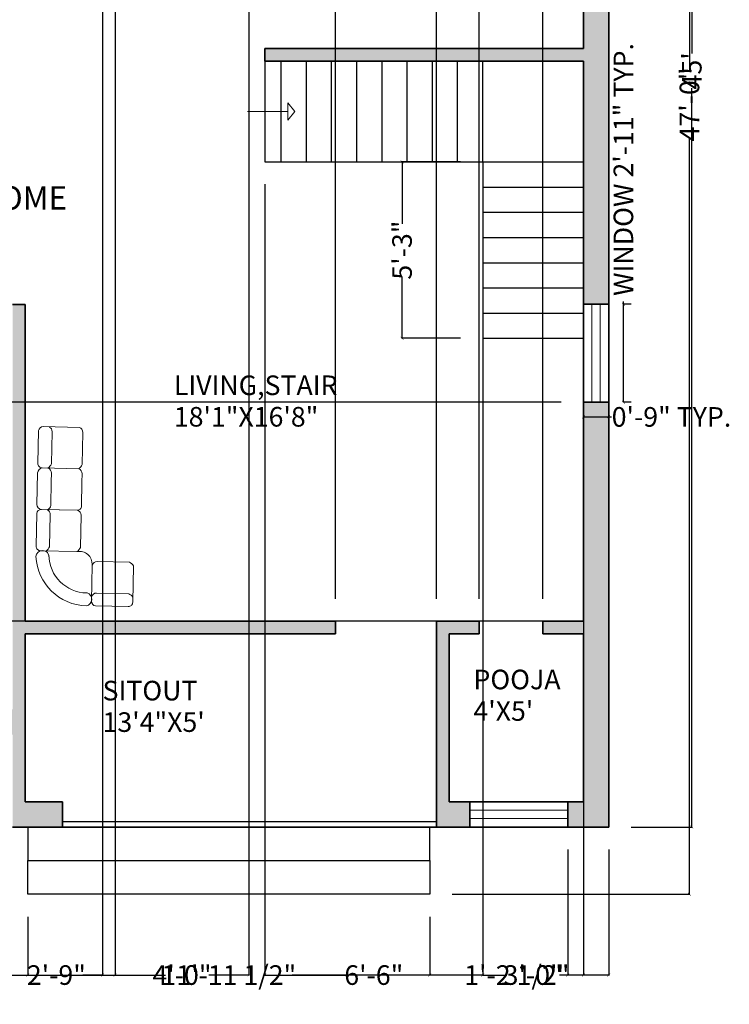
# Model space of a CAD drawing. Units: inches. Extents: x 98 to 545, y 56 to 703.
# Tile 2 of 4: x 292 to 545, y 56 to 408. Entities that reach past the tile are written whole.
import ezdxf

# ---------------------------------------------------------------- set-up
doc = ezdxf.new("R2010")
doc.units = ezdxf.units.IN
doc.header["$MEASUREMENT"] = 0
for name, color, linetype, lineweight in [('A-ANNO-DIMS', 2, 'Continuous', 18), ('A-ANNO-SYMB', 7, 'Continuous', 18), ('A-ANNO-TEXT', 7, 'Continuous', 25), ('A-AREA-IDEN', 7, 'Continuous', 25), ('A-FLOR-STRS', 7, 'Continuous', 25), ('A-GLAZ', 4, 'Continuous', 18), ('A-WALL', 7, 'Continuous', 35), ('Furniture', 7, 'Continuous', 15)]:
    doc.layers.add(name, color=color, linetype=linetype, lineweight=lineweight)
doc.layers.add('A-WALL-PATT', color=18, linetype='Continuous', lineweight=13, true_color=0x000000)
doc.styles.get("Standard").update_dxf_attribs({"font": 'arial.ttf'})
doc.dimstyles.get("Standard").update_dxf_attribs({"dimtxt": 7, "dimasz": 1, "dimexe": 0.183, "dimexo": 8, "dimgap": 0.09, "dimtad": 0, "dimdec": 4, "dimzin": 0, "dimdsep": 46, "dimlunit": 3, "dimtxsty": 'Standard', "dimblk": 'ARCHTICK', "dimcen": 0, "dimclrd": 253, "dimclre": 251, "dimadec": 0, "dimazin": 0, "dimtfac": 1, "dimtdec": 4, "dimtofl": 0, "dimtmove": 0, "dimatfit": 3, "dimfxl": 1, "dimtolj": 1, "dimtzin": 0, "dimarcsym": 0})

# ---------------------------------------------------------------- blocks, each defined once
blk = doc.blocks.new('_ArchTick')
at = {"color": 0, "linetype": 'ByBlock', "const_width": 0.15}
blk.add_lwpolyline([(-0.5, -0.5), (0.5, 0.5)], dxfattribs=at)
blk = doc.blocks.new('*D2')
at = {"layer": 'A-ANNO-DIMS', "color": 0, "lineweight": -2, "transparency": 16777216}
for p, q in [((510.36, 659.7), (532.23, 659.7)), ((532.04, 659.7), (532.04, 395.87)), ((532.04, 119.7), (532.04, 383.53)), ((510.36, 119.7), (532.23, 119.7))]:
    blk.add_line(p, q, dxfattribs=at)
at = {"layer": 'Defpoints', "color": 0, "transparency": 16777216}
for p in [(502.36, 659.7), (502.36, 119.7), (532.04, 119.7)]:
    blk.add_point(p, dxfattribs=at)
at = {"layer": 'A-ANNO-DIMS', "color": 0, "lineweight": -2, "transparency": 16777216}
for p, rotation in [((532.04, 659.7), 90), ((532.04, 119.7), 270)]:
    blk.add_blockref('_ArchTick', p, dxfattribs=dict(at, rotation=rotation))
at = {"layer": 'A-ANNO-DIMS', "color": 0, "transparency": 16777216, "insert": (532.04, 389.7), "char_height": 7, "attachment_point": 5, "rotation": 90}
blk.add_mtext("\\A1;45'", dxfattribs=at)
blk = doc.blocks.new('WIN-SASH-35IN')
for p, q in [((0, 35), (0, 0)), ((3, 35), (3, 0)), ((6, 35), (6, 0)), ((9, 0), (9, 35))]:
    blk.add_line(p, q)
blk = doc.blocks.new('*D11')
at = {"layer": 'A-ANNO-DIMS', "color": 253, "lineweight": -2, "transparency": 16777216}
for p, q in [((507.61, 306.39), (507.61, 307.39)), ((507.61, 271.39), (507.61, 306.39))]:
    blk.add_line(p, q, dxfattribs=at)
at = {"layer": 'A-ANNO-DIMS', "color": 251, "lineweight": -2, "transparency": 16777216}
for p, q in [((510.36, 306.39), (507.8, 306.39)), ((510.36, 271.39), (507.8, 271.39))]:
    blk.add_line(p, q, dxfattribs=at)
at = {"layer": 'Defpoints', "color": 0, "transparency": 16777216}
for p in [(502.36, 306.39), (507.61, 306.39), (502.36, 271.39)]:
    blk.add_point(p, dxfattribs=at)
at = {"layer": 'A-ANNO-DIMS', "color": 253, "lineweight": -2, "transparency": 16777216}
for p, rotation in [((507.61, 306.39), 90), ((507.61, 271.39), 270)]:
    blk.add_blockref('_ArchTick', p, dxfattribs=dict(at, rotation=rotation))
at = {"layer": 'A-ANNO-DIMS', "color": 0, "transparency": 16777216, "insert": (507.61, 354.48), "char_height": 7, "attachment_point": 5, "rotation": 90}
blk.add_mtext('\\A1;WINDOW 2\'-11" TYP.', dxfattribs=at)
blk = doc.blocks.new('*D12')
at = {"layer": 'A-ANNO-DIMS', "color": 253, "lineweight": -2, "transparency": 16777216}
for p, q in [((493.36, 266.14), (502.36, 266.14)), ((502.36, 266.14), (503.36, 266.14))]:
    blk.add_line(p, q, dxfattribs=at)
at = {"layer": 'A-ANNO-DIMS', "color": 251, "lineweight": -2, "transparency": 16777216}
for p, q in [((493.36, 263.39), (493.36, 265.95)), ((502.36, 263.39), (502.36, 265.95))]:
    blk.add_line(p, q, dxfattribs=at)
at = {"layer": 'Defpoints', "color": 0, "transparency": 16777216}
for p in [(493.36, 271.39), (502.36, 271.39), (502.36, 266.14)]:
    blk.add_point(p, dxfattribs=at)
at = {"layer": 'A-ANNO-DIMS', "color": 253, "lineweight": -2, "transparency": 16777216, "rotation": 180}
blk.add_blockref('_ArchTick', (493.36, 266.14), dxfattribs=at)
at = {"layer": 'A-ANNO-DIMS', "color": 253, "lineweight": -2, "transparency": 16777216}
blk.add_blockref('_ArchTick', (502.36, 266.14), dxfattribs=at)
at = {"layer": 'A-ANNO-DIMS', "color": 0, "transparency": 16777216, "insert": (524.79, 266.14), "char_height": 7, "attachment_point": 5}
blk.add_mtext('\\A1;0\'-9" TYP.', dxfattribs=at)
blk = doc.blocks.new('*D17')
at = {"layer": 'A-ANNO-DIMS', "color": 251, "lineweight": -2, "transparency": 16777216}
for p, q in [((510.36, 659.7), (531.4, 659.7)), ((446.43, 95.7), (531.4, 95.7))]:
    blk.add_line(p, q, dxfattribs=at)
at = {"layer": 'A-ANNO-DIMS', "color": 253, "lineweight": -2, "transparency": 16777216}
for p, q in [((531.21, 659.7), (531.21, 389.95)), ((531.21, 95.7), (531.21, 365.44))]:
    blk.add_line(p, q, dxfattribs=at)
at = {"layer": 'Defpoints', "color": 0, "transparency": 16777216}
for p in [(502.36, 659.7), (531.21, 659.7), (438.43, 95.7)]:
    blk.add_point(p, dxfattribs=at)
at = {"layer": 'A-ANNO-DIMS', "color": 253, "lineweight": -2, "transparency": 16777216}
for p, rotation in [((531.21, 659.7), 90), ((531.21, 95.7), 270)]:
    blk.add_blockref('_ArchTick', p, dxfattribs=dict(at, rotation=rotation))
at = {"layer": 'A-ANNO-DIMS', "color": 0, "transparency": 16777216, "insert": (531.21, 377.7), "char_height": 7, "attachment_point": 5, "rotation": 90}
blk.add_mtext('\\A1;47\'-0"', dxfattribs=at)
blk = doc.blocks.new('*D30')
at = {"layer": 'A-ANNO-DIMS', "color": 251, "lineweight": -2, "transparency": 16777216}
for p, q in [((487.75, 111.7), (487.75, 66.66)), ((502.36, 111.7), (502.36, 66.66))]:
    blk.add_line(p, q, dxfattribs=at)
at = {"layer": 'A-ANNO-DIMS', "color": 253, "lineweight": -2, "transparency": 16777216}
for p, q in [((487.75, 66.85), (486.75, 66.85)), ((502.36, 66.85), (487.75, 66.85))]:
    blk.add_line(p, q, dxfattribs=at)
at = {"layer": 'Defpoints', "color": 0, "transparency": 16777216}
for p in [(487.75, 119.7), (502.36, 119.7), (487.75, 66.85)]:
    blk.add_point(p, dxfattribs=at)
at = {"layer": 'A-ANNO-DIMS', "color": 253, "lineweight": -2, "transparency": 16777216, "rotation": 180}
blk.add_blockref('_ArchTick', (487.75, 66.85), dxfattribs=at)
at = {"layer": 'A-ANNO-DIMS', "color": 253, "lineweight": -2, "transparency": 16777216}
blk.add_blockref('_ArchTick', (502.36, 66.85), dxfattribs=at)
at = {"layer": 'A-ANNO-DIMS', "color": 0, "transparency": 16777216, "insert": (469.53, 66.85), "char_height": 7, "attachment_point": 5}
blk.add_mtext('\\A1;1\'-2 1/2"', dxfattribs=at)
blk = doc.blocks.new('*D33')
at = {"layer": 'A-ANNO-DIMS', "color": 251, "lineweight": -2, "transparency": 16777216}
for p, q in [((485.36, 271.39), (113.33, 271.39)), ((485.36, 193.2), (113.33, 193.2))]:
    blk.add_line(p, q, dxfattribs=at)
at = {"layer": 'A-ANNO-DIMS', "color": 253, "lineweight": -2, "transparency": 16777216}
for p, q in [((113.51, 271.39), (113.51, 241.7)), ((113.51, 193.2), (113.51, 222.88))]:
    blk.add_line(p, q, dxfattribs=at)
at = {"layer": 'Defpoints', "color": 0, "transparency": 16777216}
for p in [(493.36, 271.39), (113.51, 193.2), (493.36, 193.2)]:
    blk.add_point(p, dxfattribs=at)
at = {"layer": 'A-ANNO-DIMS', "color": 253, "lineweight": -2, "transparency": 16777216}
for p, rotation in [((113.51, 271.39), 90), ((113.51, 193.2), 270)]:
    blk.add_blockref('_ArchTick', p, dxfattribs=dict(at, rotation=rotation))
at = {"layer": 'A-ANNO-DIMS', "color": 0, "transparency": 16777216, "insert": (113.51, 232.29), "char_height": 7, "attachment_point": 5, "rotation": 90}
blk.add_mtext('\\A1;6\'-6"', dxfattribs=at)
blk = doc.blocks.new('*D34')
at = {"layer": 'A-ANNO-DIMS', "color": 251, "lineweight": -2, "transparency": 16777216}
for p, q in [((404.75, 201.2), (404.75, 688.73)), ((440.86, 201.2), (440.86, 688.73))]:
    blk.add_line(p, q, dxfattribs=at)
at = {"layer": 'A-ANNO-DIMS', "color": 253, "lineweight": -2, "transparency": 16777216}
for p, q in [((404.75, 688.55), (413.41, 688.55)), ((440.86, 688.55), (432.2, 688.55))]:
    blk.add_line(p, q, dxfattribs=at)
at = {"layer": 'Defpoints', "color": 0, "transparency": 16777216}
for p in [(440.86, 688.55), (404.75, 193.2), (440.86, 193.2)]:
    blk.add_point(p, dxfattribs=at)
at = {"layer": 'A-ANNO-DIMS', "color": 253, "lineweight": -2, "transparency": 16777216, "rotation": 180}
blk.add_blockref('_ArchTick', (404.75, 688.55), dxfattribs=at)
at = {"layer": 'A-ANNO-DIMS', "color": 253, "lineweight": -2, "transparency": 16777216}
blk.add_blockref('_ArchTick', (440.86, 688.55), dxfattribs=at)
at = {"layer": 'A-ANNO-DIMS', "color": 0, "transparency": 16777216, "insert": (422.81, 688.55), "char_height": 7, "attachment_point": 5}
blk.add_mtext('\\A1;3\'-0"', dxfattribs=at)
blk = doc.blocks.new('*D35')
at = {"layer": 'A-ANNO-DIMS', "color": 251, "lineweight": -2, "transparency": 16777216}
for p, q in [((456.13, 201.2), (456.13, 688.73)), ((478.77, 201.2), (478.77, 688.73))]:
    blk.add_line(p, q, dxfattribs=at)
at = {"layer": 'A-ANNO-DIMS', "color": 253, "lineweight": -2, "transparency": 16777216}
for p, q in [((456.13, 688.55), (478.77, 688.55)), ((478.77, 688.55), (479.77, 688.55))]:
    blk.add_line(p, q, dxfattribs=at)
at = {"layer": 'Defpoints', "color": 0, "transparency": 16777216}
for p in [(478.77, 688.55), (456.13, 193.2), (478.77, 193.2)]:
    blk.add_point(p, dxfattribs=at)
at = {"layer": 'A-ANNO-DIMS', "color": 253, "lineweight": -2, "transparency": 16777216, "rotation": 180}
blk.add_blockref('_ArchTick', (456.13, 688.55), dxfattribs=at)
at = {"layer": 'A-ANNO-DIMS', "color": 253, "lineweight": -2, "transparency": 16777216}
blk.add_blockref('_ArchTick', (478.77, 688.55), dxfattribs=at)
at = {"layer": 'A-ANNO-DIMS', "color": 0, "transparency": 16777216, "insert": (499.7, 688.55), "char_height": 7, "attachment_point": 5}
blk.add_mtext('\\A1;1\'-10 1/2"', dxfattribs=at)
blk = doc.blocks.new('*D36')
at = {"layer": 'A-ANNO-DIMS', "color": 251, "lineweight": -2, "transparency": 16777216}
for p, q in [((325.96, 518.2), (325.96, 66.66)), ((373.81, 518.2), (373.81, 66.66))]:
    blk.add_line(p, q, dxfattribs=at)
at = {"layer": 'A-ANNO-DIMS', "color": 253, "lineweight": -2, "transparency": 16777216}
for p, q in [((325.96, 66.85), (340.35, 66.85)), ((373.81, 66.85), (359.42, 66.85))]:
    blk.add_line(p, q, dxfattribs=at)
at = {"layer": 'Defpoints', "color": 0, "transparency": 16777216}
for p in [(325.96, 526.2), (373.81, 526.2), (373.81, 66.85)]:
    blk.add_point(p, dxfattribs=at)
at = {"layer": 'A-ANNO-DIMS', "color": 253, "lineweight": -2, "transparency": 16777216, "rotation": 180}
blk.add_blockref('_ArchTick', (325.96, 66.85), dxfattribs=at)
at = {"layer": 'A-ANNO-DIMS', "color": 253, "lineweight": -2, "transparency": 16777216}
blk.add_blockref('_ArchTick', (373.81, 66.85), dxfattribs=at)
at = {"layer": 'A-ANNO-DIMS', "color": 0, "transparency": 16777216, "insert": (349.89, 66.85), "char_height": 7, "attachment_point": 5}
blk.add_mtext('\\A1;4\'-0"', dxfattribs=at)
blk = doc.blocks.new('*D37')
at = {"layer": 'A-ANNO-DIMS', "color": 251, "lineweight": -2, "transparency": 16777216}
for p, q in [((457.36, 286.2), (457.36, 66.66)), ((493.36, 286.2), (493.36, 66.66))]:
    blk.add_line(p, q, dxfattribs=at)
at = {"layer": 'A-ANNO-DIMS', "color": 253, "lineweight": -2, "transparency": 16777216}
for p, q in [((457.36, 66.85), (465.97, 66.85)), ((493.36, 66.85), (484.76, 66.85))]:
    blk.add_line(p, q, dxfattribs=at)
at = {"layer": 'Defpoints', "color": 0, "transparency": 16777216}
for p in [(457.36, 294.2), (493.36, 294.2), (493.36, 66.85)]:
    blk.add_point(p, dxfattribs=at)
at = {"layer": 'A-ANNO-DIMS', "color": 253, "lineweight": -2, "transparency": 16777216, "rotation": 180}
blk.add_blockref('_ArchTick', (457.36, 66.85), dxfattribs=at)
at = {"layer": 'A-ANNO-DIMS', "color": 253, "lineweight": -2, "transparency": 16777216}
blk.add_blockref('_ArchTick', (493.36, 66.85), dxfattribs=at)
at = {"layer": 'A-ANNO-DIMS', "color": 0, "transparency": 16777216, "insert": (475.36, 66.85), "char_height": 7, "attachment_point": 5}
blk.add_mtext('\\A1;3\'-0"', dxfattribs=at)
blk = doc.blocks.new('*D38')
at = {"layer": 'A-ANNO-DIMS', "color": 251, "lineweight": -2, "transparency": 16777216}
for p, q in [((379.48, 349.2), (379.48, 66.66)), ((457.36, 349.2), (457.36, 66.66))]:
    blk.add_line(p, q, dxfattribs=at)
at = {"layer": 'A-ANNO-DIMS', "color": 253, "lineweight": -2, "transparency": 16777216}
for p, q in [((379.48, 66.85), (409.01, 66.85)), ((457.36, 66.85), (427.83, 66.85))]:
    blk.add_line(p, q, dxfattribs=at)
at = {"layer": 'Defpoints', "color": 0, "transparency": 16777216}
for p in [(379.48, 357.2), (457.36, 357.2), (457.36, 66.85)]:
    blk.add_point(p, dxfattribs=at)
at = {"layer": 'A-ANNO-DIMS', "color": 253, "lineweight": -2, "transparency": 16777216, "rotation": 180}
blk.add_blockref('_ArchTick', (379.48, 66.85), dxfattribs=at)
at = {"layer": 'A-ANNO-DIMS', "color": 253, "lineweight": -2, "transparency": 16777216}
blk.add_blockref('_ArchTick', (457.36, 66.85), dxfattribs=at)
at = {"layer": 'A-ANNO-DIMS', "color": 0, "transparency": 16777216, "insert": (418.42, 66.85), "char_height": 7, "attachment_point": 5}
blk.add_mtext('\\A1;6\'-6"', dxfattribs=at)
blk = doc.blocks.new('*D39')
at = {"layer": 'A-ANNO-DIMS', "color": 251, "lineweight": -2, "transparency": 16777216}
for p, q in [((449.36, 357.2), (428.33, 357.2)), ((449.36, 294.2), (428.33, 294.2))]:
    blk.add_line(p, q, dxfattribs=at)
at = {"layer": 'A-ANNO-DIMS', "color": 253, "lineweight": -2, "transparency": 16777216}
for p, q in [((428.51, 357.2), (428.51, 335.09)), ((428.51, 294.2), (428.51, 316.3))]:
    blk.add_line(p, q, dxfattribs=at)
at = {"layer": 'Defpoints', "color": 0, "transparency": 16777216}
for p in [(428.51, 357.2), (457.36, 357.2), (457.36, 294.2)]:
    blk.add_point(p, dxfattribs=at)
at = {"layer": 'A-ANNO-DIMS', "color": 253, "lineweight": -2, "transparency": 16777216}
for p, rotation in [((428.51, 357.2), 90), ((428.51, 294.2), 270)]:
    blk.add_blockref('_ArchTick', p, dxfattribs=dict(at, rotation=rotation))
at = {"layer": 'A-ANNO-DIMS', "color": 0, "transparency": 16777216, "insert": (428.51, 325.7), "char_height": 7, "attachment_point": 5, "rotation": 90}
blk.add_mtext('\\A1;5\'-3"', dxfattribs=at)
blk = doc.blocks.new('*D42')
at = {"layer": 'A-ANNO-DIMS', "color": 251, "lineweight": -2, "transparency": 16777216}
for p, q in [((288.56, 558.2), (288.56, 66.66)), ((321.46, 558.2), (321.46, 66.66))]:
    blk.add_line(p, q, dxfattribs=at)
at = {"layer": 'A-ANNO-DIMS', "color": 253, "lineweight": -2, "transparency": 16777216}
for p, q in [((288.56, 66.85), (295.56, 66.85)), ((321.46, 66.85), (314.46, 66.85))]:
    blk.add_line(p, q, dxfattribs=at)
at = {"layer": 'Defpoints', "color": 0, "transparency": 16777216}
for p in [(288.56, 566.2), (321.46, 566.2), (321.46, 66.85)]:
    blk.add_point(p, dxfattribs=at)
at = {"layer": 'A-ANNO-DIMS', "color": 253, "lineweight": -2, "transparency": 16777216, "rotation": 180}
blk.add_blockref('_ArchTick', (288.56, 66.85), dxfattribs=at)
at = {"layer": 'A-ANNO-DIMS', "color": 253, "lineweight": -2, "transparency": 16777216}
blk.add_blockref('_ArchTick', (321.46, 66.85), dxfattribs=at)
at = {"layer": 'A-ANNO-DIMS', "color": 0, "transparency": 16777216, "insert": (305.01, 66.85), "char_height": 7, "attachment_point": 5}
blk.add_mtext('\\A1;2\'-9"', dxfattribs=at)
blk = doc.blocks.new('*D43')
at = {"layer": 'A-ANNO-DIMS', "color": 251, "lineweight": -2, "transparency": 16777216}
for p, q in [((294.81, 87.7), (294.81, 66.66)), ((438.43, 87.7), (438.43, 66.66))]:
    blk.add_line(p, q, dxfattribs=at)
at = {"layer": 'A-ANNO-DIMS', "color": 253, "lineweight": -2, "transparency": 16777216}
for p, q in [((294.81, 66.85), (343.96, 66.85)), ((438.43, 66.85), (389.28, 66.85))]:
    blk.add_line(p, q, dxfattribs=at)
at = {"layer": 'Defpoints', "color": 0, "transparency": 16777216}
for p in [(294.81, 95.7), (438.43, 95.7), (438.43, 66.85)]:
    blk.add_point(p, dxfattribs=at)
at = {"layer": 'A-ANNO-DIMS', "color": 253, "lineweight": -2, "transparency": 16777216, "rotation": 180}
blk.add_blockref('_ArchTick', (294.81, 66.85), dxfattribs=at)
at = {"layer": 'A-ANNO-DIMS', "color": 253, "lineweight": -2, "transparency": 16777216}
blk.add_blockref('_ArchTick', (438.43, 66.85), dxfattribs=at)
at = {"layer": 'A-ANNO-DIMS', "color": 0, "transparency": 16777216, "insert": (366.62, 66.85), "char_height": 7, "attachment_point": 5}
blk.add_mtext('\\A1;11\'-11 1/2"', dxfattribs=at)
blk = doc.blocks.new('*D47')
at = {"layer": 'A-ANNO-DIMS', "color": 251, "lineweight": -2, "transparency": 16777216}
for p, q in [((271.36, 409.7), (271.36, 688.73)), ((275.86, 409.7), (275.86, 688.73))]:
    blk.add_line(p, q, dxfattribs=at)
at = {"layer": 'A-ANNO-DIMS', "color": 253, "lineweight": -2, "transparency": 16777216}
for p, q in [((271.36, 688.55), (275.86, 688.55)), ((275.86, 688.55), (276.86, 688.55))]:
    blk.add_line(p, q, dxfattribs=at)
at = {"layer": 'Defpoints', "color": 0, "transparency": 16777216}
for p in [(275.86, 688.55), (271.36, 401.7), (275.86, 401.7)]:
    blk.add_point(p, dxfattribs=at)
at = {"layer": 'A-ANNO-DIMS', "color": 253, "lineweight": -2, "transparency": 16777216, "rotation": 180}
blk.add_blockref('_ArchTick', (271.36, 688.55), dxfattribs=at)
at = {"layer": 'A-ANNO-DIMS', "color": 253, "lineweight": -2, "transparency": 16777216}
blk.add_blockref('_ArchTick', (275.86, 688.55), dxfattribs=at)
at = {"layer": 'A-ANNO-DIMS', "color": 0, "transparency": 16777216, "insert": (294.41, 688.55), "char_height": 7, "attachment_point": 5}
blk.add_mtext('\\A1;0\'-4 1/2"', dxfattribs=at)

msp = doc.modelspace()

# ---------------------------------------------------------------- hatches: boundary and pattern name
at = {"layer": 'A-WALL-PATT'}
h = msp.add_hatch(color=256, dxfattribs=at)
h.dxf.hatch_style = 1
h.paths.add_polyline_path([(173.39577, 659.69681), (142.36469, 659.69681), (142.36469, 612.44216), (151.36469, 612.44216), (151.36469, 650.69681), (173.39577, 650.69681)])
h.paths.add_polyline_path([(282.86266, 659.69681), (220.39577, 659.69681), (220.39577, 650.69681), (271.36469, 650.69681), (271.36469, 566.19681), (275.86469, 566.19681), (288.55623, 566.19681), (288.55623, 570.69681), (275.86469, 570.69681), (275.86469, 650.69681), (282.86266, 650.69681)])
h.paths.add_polyline_path([(358.82163, 659.69681), (312.86266, 659.69681), (312.86266, 650.69681), (321.46469, 650.69681), (321.46469, 570.69681), (321.46469, 566.19681), (321.46469, 530.69681), (321.46469, 526.19681), (325.96469, 526.19681), (325.96469, 530.69681), (325.96469, 650.69681), (358.82163, 650.69681)])
h.paths.add_polyline_path([(451.98971, 659.69681), (405.82163, 659.69681), (405.82163, 650.69681), (435.16469, 650.69681), (435.16469, 570.08746), (439.66469, 570.08746), (439.66469, 650.69681), (451.98971, 650.69681)])
h.paths.add_polyline_path([(502.36469, 659.69681), (481.98971, 659.69681), (481.98971, 650.69681), (493.36469, 650.69681), (493.36469, 614.57752), (502.36469, 614.57752)])
h.paths.add_polyline_path([(502.36469, 579.57752), (493.36469, 579.57752), (493.36469, 530.69681), (439.66469, 530.69681), (435.16469, 530.69681), (373.81242, 530.69681), (373.81242, 526.19681), (493.36469, 526.19681), (493.36469, 480.62471), (502.36469, 480.62471)])
h.paths.add_polyline_path([(502.36469, 445.62471), (493.36469, 445.62471), (493.36469, 406.19681), (493.36469, 401.69681), (493.36469, 397.69681), (379.47742, 397.69681), (379.47742, 393.19681), (493.36469, 393.19681), (493.36469, 306.38501), (502.36469, 306.38501)])
h.paths.add_polyline_path([(502.36469, 271.385), (493.36469, 271.385), (493.36469, 193.19681), (478.76571, 193.19681), (478.76571, 188.69681), (493.36469, 188.69681), (493.36469, 128.69681), (487.75103, 128.69681), (487.75103, 119.69681), (502.36469, 119.69681)])
h.paths.add_polyline_path([(452.75103, 128.69681), (445.36469, 128.69681), (445.36469, 188.69681), (456.12508, 188.69681), (456.12508, 193.19681), (440.86469, 193.19681), (440.86469, 119.69681), (452.75103, 119.69681)])
h.paths.add_polyline_path([(307.21941, 128.69681), (293.86469, 128.69681), (293.86469, 188.69681), (404.74827, 188.69681), (404.74827, 193.19681), (293.86469, 193.19681), (293.86469, 306.29681), (289.36469, 306.29681), (289.36469, 119.69681), (307.21941, 119.69681)])
h.paths.add_polyline_path([(289.36469, 161.69681), (238.02122, 161.69681), (238.02122, 152.69681), (289.36469, 152.69681)])
h.paths.add_polyline_path([(191.02122, 161.69681), (151.36469, 161.69681), (151.36469, 191.65928), (142.36469, 191.65928), (142.36469, 152.69681), (151.36469, 152.69681), (191.02122, 152.69681)])
h.paths.add_polyline_path([(151.36469, 306.29681), (151.36469, 308.54862), (142.36469, 308.54862), (142.36469, 238.65928), (151.36469, 238.65928)])
h.paths.add_polyline_path([(230.26469, 401.69681), (230.26469, 406.19681), (182.81458, 406.19681), (182.81458, 401.69681), (225.76469, 401.69681), (225.76469, 358.49681), (151.36469, 358.49681), (151.36469, 368.55378), (142.36469, 368.55378), (142.36469, 338.54862), (151.36469, 338.54862), (151.36469, 353.99681), (225.76469, 353.99681), (225.76469, 310.79681), (180.84919, 310.79681), (180.84919, 306.29681), (230.26469, 306.29681)])
h.paths.add_polyline_path([(151.36469, 442.07867), (142.36469, 442.07867), (142.36469, 398.55378), (151.36469, 398.55378), (151.36469, 401.69681)])
h.paths.add_polyline_path([(151.36469, 526.19681), (271.36469, 526.19681), (271.36469, 406.19681), (271.36469, 401.69681), (275.86469, 401.69681), (275.86469, 406.19681), (275.86469, 526.19681), (275.86469, 530.69681), (271.36469, 530.69681), (151.36469, 530.69681), (151.36469, 565.44216), (142.36469, 565.44216), (142.36469, 489.07867), (151.36469, 489.07867)])

# ---------------------------------------------------------------- linework, layer by layer
at = {"layer": 'A-ANNO-SYMB'}
for p, q in [((390.21777, 375.19681), (387.6515, 378.31614)), ((387.6515, 378.31614), (387.6515, 375.19681)), ((373.3537, 375.19681), (387.6515, 375.19681)), ((390.21777, 375.19681), (387.6515, 372.07747)), ((387.6515, 372.07747), (387.6515, 375.19681))]:
    msp.add_line(p, q, dxfattribs=at)
at = {"layer": 'A-FLOR-STRS'}
for p, q in [((379.47742, 393.19681), (379.47742, 357.19681)), ((385.36469, 357.19681), (385.36469, 393.19681)), ((394.36469, 357.19681), (394.36469, 393.19681)), ((403.36469, 357.19681), (403.36469, 393.19681)), ((412.36469, 357.19681), (412.36469, 393.19681)), ((421.36469, 357.19681), (421.36469, 393.19681)), ((430.36469, 357.19681), (430.36469, 393.19681)), ((439.36469, 357.19681), (439.36469, 393.19681)), ((448.36469, 357.19681), (448.36469, 393.19681)), ((457.36469, 357.19681), (457.36469, 393.19681)), ((379.47742, 357.19681), (493.36469, 357.19681)), ((457.36469, 357.19681), (457.36469, 294.19681)), ((457.36469, 348.19681), (493.36469, 348.19681)), ((457.36469, 339.19681), (493.36469, 339.19681)), ((457.36469, 330.19681), (493.36469, 330.19681)), ((457.36469, 321.19681), (493.36469, 321.19681)), ((457.36469, 312.19681), (493.36469, 312.19681)), ((457.36469, 303.19681), (493.36469, 303.19681)), ((457.36469, 294.19681), (493.36469, 294.19681)), ((294.80527, 119.69681), (294.80527, 107.69681)), ((307.21941, 121.69681), (440.86469, 121.69681)), ((438.43213, 107.69681), (438.43213, 119.69681)), ((294.80527, 107.69681), (438.43213, 107.69681)), ((294.80527, 95.69681), (294.80527, 107.69681)), ((438.43213, 107.69681), (438.43213, 95.69681)), ((438.43213, 95.69681), (294.80527, 95.69681))]:
    msp.add_line(p, q, dxfattribs=at)
at = {"layer": 'A-WALL'}
for p, q in [((502.36469, 119.69681), (502.36469, 659.69681)), ((493.36469, 406.19681), (493.36469, 526.19681)), ((493.36469, 401.69681), (493.36469, 406.19681)), ((493.36469, 397.69681), (493.36469, 401.69681)), ((379.47742, 397.69681), (493.36469, 397.69681)), ((379.47742, 397.69681), (379.47742, 393.19681)), ((379.47742, 393.19681), (493.36469, 393.19681)), ((493.36469, 193.19681), (493.36469, 393.19681)), ((293.86469, 306.29681), (289.36469, 306.29681)), ((293.86469, 306.29681), (293.86469, 193.19681)), ((502.36469, 306.38501), (493.36469, 306.38501)), ((493.36469, 271.385), (502.36469, 271.385)), ((293.86469, 193.19681), (404.74827, 193.19681)), ((404.74827, 193.19681), (404.74827, 188.69681)), ((440.86469, 119.69681), (440.86469, 193.19681)), ((440.86469, 193.19681), (456.12508, 193.19681)), ((456.12508, 188.69681), (456.12508, 193.19681)), ((478.76571, 188.69681), (478.76571, 193.19681)), ((478.76571, 193.19681), (493.36469, 193.19681)), ((293.86469, 188.69681), (404.74827, 188.69681)), ((293.86469, 188.69681), (293.86469, 128.69681)), ((445.36469, 128.69681), (445.36469, 188.69681)), ((445.36469, 188.69681), (456.12508, 188.69681)), ((478.76571, 188.69681), (493.36469, 188.69681)), ((493.36469, 128.69681), (493.36469, 188.69681)), ((293.86469, 128.69681), (307.21941, 128.69681)), ((307.21941, 128.69681), (307.21941, 119.69681)), ((445.36469, 128.69681), (493.36469, 128.69681)), ((452.75103, 128.69681), (452.75103, 119.69681)), ((487.75103, 119.69681), (487.75103, 128.69681)), ((289.36469, 119.69681), (502.36469, 119.69681))]:
    msp.add_line(p, q, dxfattribs=at)
at = {"layer": 'Furniture'}
for p, q in [((298.63616, 261.22932), (298.38808, 249.54981)), ((313.226, 262.3968), (300.27769, 262.67184)), ((303.22838, 249.37984), (303.4722, 260.85798)), ((314.21982, 249.14637), (314.46363, 260.62451)), ((298.31678, 246.19363), (298.07582, 234.84973)), ((299.96543, 247.97176), (312.97941, 247.62817)), ((302.98037, 234.54409), (303.16287, 243.13592)), ((303.16287, 243.13592), (303.22418, 246.02223)), ((313.97181, 234.31062), (314.15431, 242.90244)), ((314.15431, 242.90244), (314.21562, 245.78876)), ((299.51473, 233.07317), (312.39595, 232.79955)), ((312.59728, 232.79808), (299.64897, 233.07312)), ((298.00745, 231.63061), (297.75936, 219.95109)), ((302.59967, 219.78113), (302.84348, 231.25927)), ((313.5911, 219.54765), (313.83491, 231.02579)), ((299.33671, 218.37305), (312.35069, 218.02946)), ((331.09751, 214.23754), (319.61936, 214.48135)), ((317.84707, 213.24372), (317.57203, 200.29541)), ((332.6157, 212.99713), (332.27211, 199.98316)), ((316.02137, 203.27911), (315.86446, 203.28245)), ((317.60809, 201.99312), (317.60711, 201.94682)), ((330.85853, 202.98694), (319.38039, 203.23075)), ((319.01455, 198.65389), (330.69406, 198.4058))]:
    msp.add_line(p, q, dxfattribs=at)
for centre, radius, start, end in [((300.24336, 261.05566), 1.61655, 88.783137, 173.8328903), ((301.64015, 260.8969), 1.83246, 358.783137, 62.8574556), ((312.63158, 260.66342), 1.83246, 358.783137, 71.0719068), ((300.5577, 245.76926), 2.28074, 105.0511292, 169.276828), ((299.93328, 249.51699), 1.54556, 178.783137, 271.1919529), ((299.79157, 250.922), 3.76696, 305.666939, 335.8333646), ((301.29847, 246.06314), 1.92615, 358.783137, 69.0242602), ((310.783, 250.68853), 3.76696, 305.666939, 335.8333646), ((312.2899, 245.82966), 1.92615, 358.783137, 69.0242602), ((299.61464, 231.45694), 1.61655, 88.783137, 173.8328903), ((299.8456, 234.81214), 1.77017, 178.783137, 259.2272933), ((301.01143, 231.29818), 1.83246, 358.783137, 62.8574556), ((301.43729, 234.57609), 1.54341, 285.5408754, 358.8120982), ((312.42873, 234.34262), 1.54341, 268.783137, 358.8120982), ((312.00286, 231.06471), 1.83246, 358.783137, 71.0719068), ((300.03988, 216.14235), 2.34094, 356.795265, 176.795265), ((299.30456, 219.91827), 1.54556, 178.783137, 271.1919529), ((299.16285, 221.32329), 3.76696, 305.666939, 335.8333646), ((310.15428, 221.08981), 3.76696, 305.666939, 335.8333646), ((313.18783, 213.51232), 4.63077, 358.783137, 99.3837611), ((316.15958, 217.17584), 18.47811, 182.7701723, 268.7314166), ((316.15958, 217.17584), 13.89653, 181.6990742, 268.783137), ((319.58045, 212.6493), 1.83246, 88.783137, 161.0719068), ((329.55534, 210.80072), 3.76696, 35.666939, 65.8333646), ((315.29, 201.02596), 2.36889, 281.2092121, 72.0166253), ((319.34147, 201.3987), 1.83246, 88.783137, 161.0719068), ((329.31636, 199.55012), 3.76696, 35.666939, 65.8333646), ((319.18821, 200.26108), 1.61655, 178.783137, 263.8328903), ((330.72688, 199.95101), 1.54556, 268.783137, 1.1919529)]:
    msp.add_arc(centre, radius, start, end, dxfattribs=at)

# ---------------------------------------------------------------- block references
at = {"layer": 'A-GLAZ'}
msp.add_blockref('WIN-SASH-35IN', (493.365, 271.385), dxfattribs=at)
at = {"layer": 'A-GLAZ', "rotation": 89.99999999999969}
msp.add_blockref('WIN-SASH-35IN', (487.75104, 119.69711), dxfattribs=at)

# ---------------------------------------------------------------- texts
at = {"layer": 'A-ANNO-TEXT'}
msp.add_text('HOME', height=8.320668, dxfattribs=at).set_placement((276.29482, 340.16056))
at = {"layer": 'A-AREA-IDEN'}
for s, p in [('LIVING,STAIR', (346.97361, 273.93277)), ('18\'1"X16\'8"', (346.97361, 262.68789)), ('POOJA', (454.02372, 168.88786)), ('SITOUT ', (321.50558, 164.91482)), ("4'X5'", (454.02372, 157.64297)), ('13\'4"X5\'', (321.50558, 153.66993))]:
    msp.add_text(s, height=7, dxfattribs=at).set_placement(p)

# ---------------------------------------------------------------- dimensions: what is measured, and where the dimension line sits
at = {"layer": 'A-ANNO-DIMS'}
for base, p1, p2, picture, middle in [((275.86469, 688.54681), (271.36469, 401.69681), (275.86469, 401.69681), '*D47', (294.41411, 688.54681)), ((478.76571, 688.54681), (456.12509, 193.19681), (478.76571, 193.19681), '*D35', (499.70496, 688.54681)), ((440.86469, 688.54681), (404.74827, 193.19681), (440.86469, 193.19681), '*D34', (422.80648, 688.54681)), ((321.46469, 66.84681), (288.55623, 566.19681), (321.46469, 566.19681), '*D42', (305.01046, 66.84681)), ((373.81242, 66.84681), (325.96469, 526.19681), (373.81242, 526.19681), '*D36', (349.88856, 66.84681)), ((457.36469, 66.84681), (379.47742, 357.19681), (457.36469, 357.19681), '*D38', (418.42106, 66.84681)), ((493.36469, 66.84681), (457.36469, 294.19681), (493.36469, 294.19681), '*D37', (475.36469, 66.84681)), ((487.75104, 66.84681), (502.36469, 119.69681), (487.75104, 119.69681), '*D30', (469.53109, 66.84681)), ((438.43212, 66.84681), (294.80527, 95.69681), (438.43212, 95.69681), '*D43', (366.6187, 66.84681))]:
    dim = msp.add_linear_dim(base=base, p1=p1, p2=p2, dimstyle='Standard', override={"dimdec": 1, "dimlfac": 1, "dimrnd": 0, "dimzin": 1, "dimdsep": 46, "dimlunit": 4, "dimfrac": 2}, dxfattribs=at)
    dim.commit()
    dim.dimension.update_dxf_attribs({"geometry": picture, "text_midpoint": middle})
for base, p1, p2, override, picture, middle in [((531.21469, 659.69681), (438.43212, 95.69681), (502.36469, 659.69681), {"dimdec": 1, "dimlfac": 1, "dimrnd": 0, "dimzin": 1, "dimdsep": 46, "dimlunit": 4, "dimfrac": 2}, '*D17', (531.21469, 377.69681)), ((532.04321, 119.69681), (502.36469, 659.69681), (502.36469, 119.69681), {"dimclrd": 0, "dimclre": 0, "dimclrt": 0}, '*D2', (532.04321, 389.69681)), ((428.51469, 357.19681), (457.36469, 294.19681), (457.36469, 357.19681), {"dimdec": 1, "dimlfac": 1, "dimrnd": 0, "dimzin": 1, "dimdsep": 46, "dimlunit": 4, "dimfrac": 2}, '*D39', (428.51469, 325.69681)), ((113.51469, 193.19681), (493.36469, 271.385), (493.36469, 193.19681), {"dimdec": 1, "dimlfac": 1, "dimrnd": 0, "dimzin": 1, "dimdsep": 46, "dimlunit": 4, "dimfrac": 2}, '*D33', (113.51469, 232.29091))]:
    dim = msp.add_linear_dim(base=base, p1=p1, p2=p2, angle=90, dimstyle='Standard', override=override, dxfattribs=at)
    dim.commit()
    dim.dimension.update_dxf_attribs({"geometry": picture, "text_midpoint": middle})
dim = msp.add_linear_dim(base=(507.61469, 306.38501), p1=(502.36469, 271.385), p2=(502.36469, 306.38501), angle=90, text='WINDOW <> TYP.', dimstyle='Standard', override={"dimdec": 1, "dimlfac": 1, "dimrnd": 0, "dimzin": 1, "dimdsep": 46, "dimlunit": 4, "dimfrac": 2}, dxfattribs=at)
dim.commit()
dim.dimension.update_dxf_attribs({"geometry": '*D11', "text_midpoint": (507.61469, 354.48387)})
dim = msp.add_linear_dim(base=(502.36469, 266.13501), p1=(493.36469, 271.385), p2=(502.36469, 271.385), text='<> TYP.', dimstyle='Standard', override={"dimdec": 1, "dimlfac": 1, "dimrnd": 0, "dimzin": 1, "dimdsep": 46, "dimlunit": 4, "dimfrac": 2}, dxfattribs=at)
dim.commit()
dim.dimension.update_dxf_attribs({"geometry": '*D12', "text_midpoint": (524.78894, 266.13501)})

doc.saveas('drawing.dxf')
